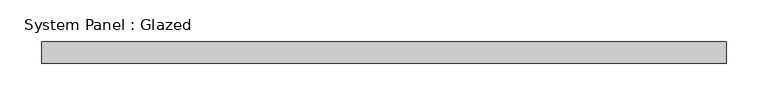
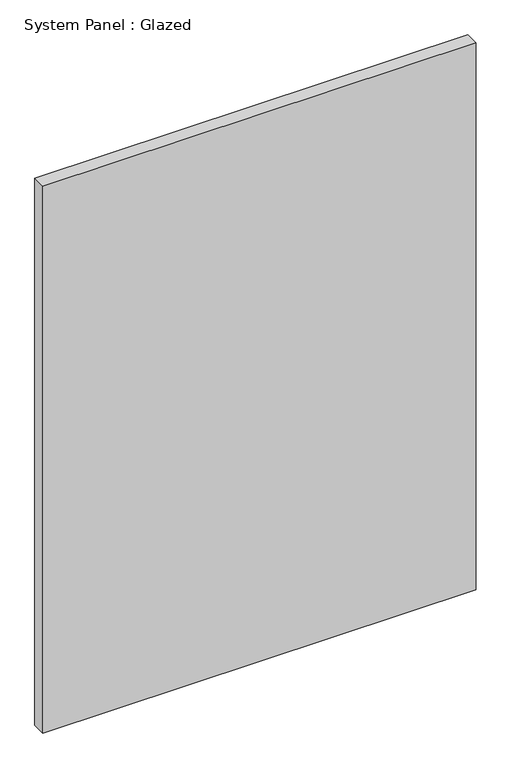
"""IFC4 building model written with IfcOpenShell, lengths in millimetres: plate geometry, System Panel : Glazed."""

from ifc_helpers import new_model, si_unit, origin, origin_with_axes, place, context, project, spatial, polyline, outline, extrude, source, transform, mapped, element, save


def system_panel_glazed_7cebc396(model_context):
    return source(origin(), model_context, "Body", "SweptSolid", [
        extrude(outline(polyline([(409.4264909, 19.05), (-409.4264909, 19.05), (-409.4264909, 44.45), (409.4264909, 44.45), (409.4264909, 19.05)])), origin_with_axes(), (0.0, 0.0, 1.0), 1092.2),
    ])


if __name__ == "__main__":
    model = new_model("IFC4")
    model_context = context("Model", 3, world=origin())
    ifc_project = project(units=[si_unit("LENGTHUNIT", "METRE", prefix="MILLI")], contexts=[model_context])
    site = spatial("IfcSite", under=ifc_project)
    building = spatial("IfcBuilding", under=site)
    placement = place(None, origin())
    system_panel_glazed_shape = system_panel_glazed_7cebc396(model_context)
    element("IfcPlate", 1, ObjectType="System Panel : Glazed", at=placement, inside=building, context=model_context, shape_type="MappedRepresentation", body=[
        mapped(system_panel_glazed_shape, transform((0.0, 0.0, 0.0), x_axis=(1.0, 0.0, 0.0), y_axis=(0.0, 1.0, 0.0), z_axis=(0.0, 0.0, 1.0))),
    ])
    save(model, "model.ifc")

# Revit data of these elements
# Type "System Panel : Glazed"
#   Construction Type Id = "GSP4R"
#   Analytic Construction = "1/8 in Pilkington single glazing"
#   Visual Light Transmittance = 0.9
#   Solar Heat Gain Coefficient = 0.86
#   Heat Transfer Coefficient (U) = 1.18115 BTU/(h·ft²·°F)
#   Define Thermal Properties by = 1
# Element 1 (IfcPlate, "System Panel : Glazed")
#   Materials on its faces: "Glass"
# Materials
#   "Glass": class "Glass", colour RGB 0 128 192, transparency 0.75, Description = "Soda Lime Glass", Cost = 0
